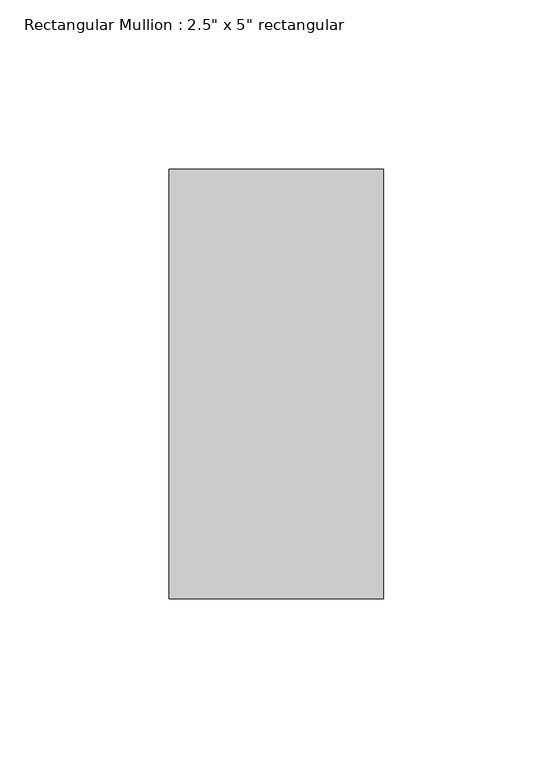
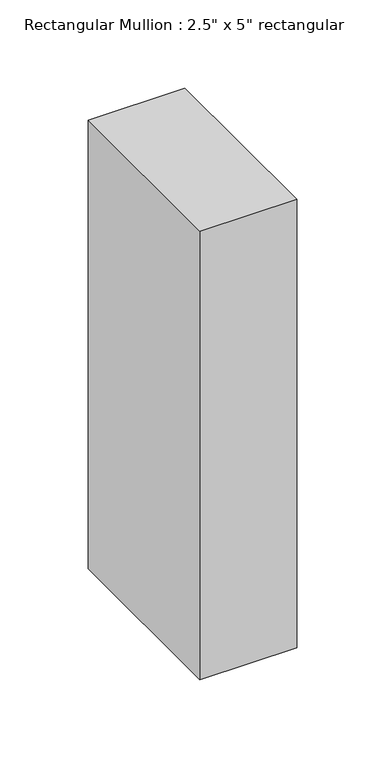
"""IFC4 building model written with IfcOpenShell, lengths in millimetres: member geometry."""

from ifc_helpers import new_model, si_unit, frame, origin, place, context, project, spatial, polyline, outline, extrude, source, transform, mapped, element, save


def member_5ad95953(model_context):
    return source(origin(), model_context, "Body", "SweptSolid", [
        extrude(outline(polyline([(0.0, 63.5), (0.0, -63.5), (-63.5, -63.5), (-63.5, 63.5), (0.0, 63.5)])), frame((0.0, 0.0, -311.15), z_axis=(0.0, 0.0, 1.0), x_axis=(1.0, 0.0, 0.0)), (0.0, 0.0, 1.0), 311.15),
    ])


if __name__ == "__main__":
    model = new_model("IFC4")
    model_context = context("Model", 3, world=origin())
    ifc_project = project(units=[si_unit("LENGTHUNIT", "METRE", prefix="MILLI")], contexts=[model_context])
    site = spatial("IfcSite", under=ifc_project)
    building = spatial("IfcBuilding", under=site)
    placement = place(None, origin())
    member_shape = member_5ad95953(model_context)
    element("IfcMember", 1, ObjectType="Rectangular Mullion : 2.5\" x 5\" rectangular", at=placement, inside=building, context=model_context, shape_type="MappedRepresentation", body=[
        mapped(member_shape, transform((0.0, 0.0, 0.0), x_axis=(1.0, 0.0, 0.0), y_axis=(0.0, 1.0, 0.0), z_axis=(0.0, 0.0, 1.0))),
    ])
    save(model, "model.ifc")

# Revit data of these elements
# Type "Rectangular Mullion : 2.5\" x 5\" rectangular"
#   built-in parameter 1007304 = 0.416667 (stored number, unit not read)
#   built-in parameter 1007301 = 0.104167 (stored number, unit not read)
#   built-in parameter 1007300 = 0.104167 (stored number, unit not read)
# Element 1 (IfcMember, "Rectangular Mullion : 2.5\" x 5\" rectangular")
#   Materials on its faces: "Aluminum"
# Materials
#   "Aluminum": class "Metal", colour RGB 247 247 247, transparency 0, Description = "Aluminum 6061", Cost = 0
